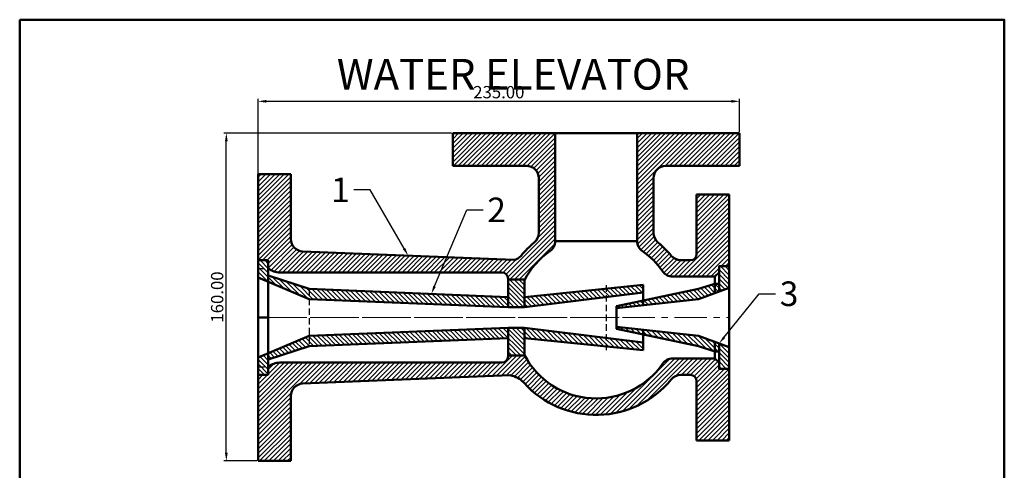
# Model space of a CAD drawing. Units: millimetres. Extents: x 39 to 520, y -165 to 464.
# Tile 4 of 4: x 39 to 520, y 244 to 464. Entities that reach past the tile are written whole.
import ezdxf
from ezdxf import colors
from ezdxf.entities.mleader import LeaderData, LeaderLine
from ezdxf.math import Vec2, Vec3

# ---------------------------------------------------------------- set-up
doc = ezdxf.new("R2010")
doc.units = ezdxf.units.MM
doc.header["$LTSCALE"] = 0.5
doc.linetypes.add('CENTER', pattern=[50.8, 31.75, -6.35, 6.35, -6.35])
doc.linetypes.add('DASHED', pattern=[19.05, 12.7, -6.35])
for name, color, linetype, lineweight in [('M-CNTR', 1, 'CENTER', 18), ('M-DIMS', 2, 'Continuous', 25), ('M-HATC', 8, 'Continuous', 18), ('M-HIDN', 6, 'DASHED', 25), ('M-OUTL', 7, 'Continuous', 50), ('M-TEXT', 3, 'Continuous', 25), ('M-TTLB', 7, 'Continuous', 50)]:
    doc.layers.add(name, color=color, linetype=linetype, lineweight=lineweight)
doc.styles.get("Standard").update_dxf_attribs({"font": 'arial.ttf'})
doc.dimstyles.new('ISO-25', dxfattribs={"dimtxt": 6, "dimasz": 4, "dimexe": 1.25, "dimexo": 0.625, "dimtad": 1, "dimtoh": 1, "dimdec": 1, "dimtxsty": 'Standard', "dimcen": 2.5, "dimadec": 0, "dimazin": 0, "dimtfac": 1, "dimtdec": 1, "dimtofl": 0, "dimtmove": 0, "dimatfit": 3, "dimfxl": 1, "dimarcsym": 0})

# ---------------------------------------------------------------- blocks, each defined once
blk = doc.blocks.new('*D65')
at = {"layer": 'Defpoints', "color": 0, "ltscale": 0.5, "transparency": 16777216}
for p in [(390.62, 424.1), (390.62, 408.6), (155.62, 248.6)]:
    blk.add_point(p, dxfattribs=at)
at = {"layer": 'M-DIMS', "color": 0, "lineweight": -2, "ltscale": 0.5, "transparency": 16777216}
for p, q in [((155.62, 249.23), (155.62, 425.35)), ((159.62, 424.1), (386.62, 424.1)), ((390.62, 409.23), (390.62, 425.35))]:
    blk.add_line(p, q, dxfattribs=at)
at = {"layer": 'M-DIMS', "color": 0, "ltscale": 0.5, "transparency": 16777216}
for points in [[(159.62, 424.77), (159.62, 423.44), (155.62, 424.1)], [(386.62, 424.77), (386.62, 423.44), (390.62, 424.1)]]:
    blk.add_solid(points, dxfattribs=at)
at = {"layer": 'M-DIMS', "color": 0, "ltscale": 0.5, "transparency": 16777216, "insert": (273.12, 427.79), "char_height": 6, "attachment_point": 5}
blk.add_mtext('235.00', dxfattribs=at)
blk = doc.blocks.new('*D66')
at = {"layer": 'Defpoints', "color": 0, "ltscale": 0.5, "transparency": 16777216}
for p in [(140.12, 408.6), (250.62, 408.6), (155.62, 248.6)]:
    blk.add_point(p, dxfattribs=at)
at = {"layer": 'M-DIMS', "color": 0, "lineweight": -2, "ltscale": 0.5, "transparency": 16777216}
for p, q in [((249.99, 408.6), (138.87, 408.6)), ((140.12, 252.6), (140.12, 404.6)), ((154.99, 248.6), (138.87, 248.6))]:
    blk.add_line(p, q, dxfattribs=at)
at = {"layer": 'M-DIMS', "color": 0, "ltscale": 0.5, "transparency": 16777216}
for points in [[(139.45, 404.6), (140.79, 404.6), (140.12, 408.6)], [(139.45, 252.6), (140.79, 252.6), (140.12, 248.6)]]:
    blk.add_solid(points, dxfattribs=at)
at = {"layer": 'M-DIMS', "color": 0, "ltscale": 0.5, "transparency": 16777216, "insert": (136.43, 328.6), "char_height": 6, "attachment_point": 5, "rotation": 90}
blk.add_mtext('160.00', dxfattribs=at)

msp = doc.modelspace()

# ---------------------------------------------------------------- hatches: boundary and pattern name
at = {"layer": 'M-HATC', "ltscale": 0.5}
h = msp.add_hatch(dxfattribs=at)
h.set_pattern_fill('ANSI31', color=256, scale=0.5)
h.set_pattern_definition([(45, (679.1988, 50.7649), (-1.122532, 1.122532), [])])
h.paths.add_polyline_path([(298.0475, 351.0177, 0.24539268), (300.6189, 355.9416), (300.6189, 408.6019), (250.6189, 408.6019), (250.6189, 392.6019), (286.6189, 392.6019, -0.41421356), (292.6189, 386.6019), (292.6189, 359.9087, -0.22417658), (290.432, 355.2762, 0.04839978), (283.9447, 348.7888, -0.17668241), (280.4018, 346.7017), (177.3764, 350.869, -0.40242153), (171.6189, 356.8641), (171.6189, 388.6019), (155.6189, 388.6019), (155.6189, 346.6019), (160.6189, 346.6019), (160.6189, 342.6019, 0.17132661), (166.3069, 340.6019), (274.6189, 340.6019, -0.41421356), (277.6189, 337.6019), (277.6189, 337.1019), (285.7191, 337.1019, -0.11934263)])
h.paths.add_polyline_path([(285.7191, 300.1019), (277.6189, 300.1019), (277.6189, 299.6019, -0.41421356), (274.6189, 296.6019), (166.2844, 296.6019, 0.17068716), (160.6189, 294.6019), (160.6189, 291.1019), (160.6189, 290.6019), (155.6189, 290.6019), (155.6189, 248.6019), (171.6189, 248.6019), (171.6189, 280.3397, -0.40242153), (177.3764, 286.3348), (278.5991, 290.4293, -0.16745848), (285.4544, 286.6692, 0.4573052), (357.2932, 288.415, -0.22417658), (361.9257, 290.6019), (366.6189, 290.6019, -0.41421356), (369.6189, 287.6019), (369.6189, 258.6019), (385.6189, 258.6019), (385.6189, 293.6019), (380.6189, 293.6019), (380.6189, 296.6019), (378.6189, 298.6019), (357.9586, 298.6019, 0.24539268), (353.0347, 296.0305, -0.56130329)])
h.paths.add_polyline_path([(385.6189, 378.6019), (369.6189, 378.6019), (369.6189, 349.6019, -0.41421356), (366.6189, 346.6019), (361.9257, 346.6019, -0.22417658), (357.2932, 348.7888, 0.04839978), (350.8059, 355.2762, -0.22417658), (348.6189, 359.9087), (348.6189, 386.6019, -0.41421356), (354.6189, 392.6019), (390.6189, 392.6019), (390.6189, 408.6019), (340.6189, 408.6019), (340.6189, 355.9416, 0.24539268), (343.1904, 351.0177, -0.08880867), (353.0347, 341.1734, 0.24539268), (357.9586, 338.6019), (378.6189, 338.6019), (380.6189, 340.6019), (380.6189, 343.6019), (385.6189, 343.6019)])
h = msp.add_hatch(dxfattribs=at)
h.set_pattern_fill('ANSI31', color=256, scale=0.5, angle=90)
h.set_pattern_definition([(135, (679.1988, 50.7649), (-1.122532, -1.122532), [])])
h.paths.add_polyline_path([(277.6189, 308.6019), (277.6189, 313.6019), (180.6189, 309.6019), (180.6189, 304.6019)])
h.paths.add_polyline_path([(180.6189, 309.6019), (160.6189, 301.2019), (160.6189, 298.1019), (180.6189, 304.6019)])
h.paths.add_polyline_path([(160.6189, 298.1019), (160.6189, 301.2019), (155.6189, 299.1019), (155.6189, 294.6019), (160.6189, 294.6019)])
h.paths.add_polyline_path([(160.6189, 294.6019), (155.6189, 294.6019), (155.6189, 291.1019), (155.6189, 290.6019), (160.6189, 290.6019)])
h.paths.add_polyline_path([(160.6189, 342.6019), (155.6189, 342.6019), (155.6189, 338.1019), (160.6189, 336.0019)])
h.paths.add_polyline_path([(160.6189, 346.1019), (160.6189, 346.6019), (155.6189, 346.6019), (155.6189, 342.6019), (160.6189, 342.6019)])
h.paths.add_polyline_path([(160.6189, 339.1019), (160.6189, 336.0019), (180.6189, 327.6019), (180.6189, 332.6019)])
h.paths.add_polyline_path([(180.6189, 332.6019), (180.6189, 327.6019), (277.6189, 323.6019), (277.6189, 328.6019)])
h.paths.add_polyline_path([(325.6189, 328.6019), (325.6189, 332.7399), (285.6189, 328.6019), (285.6189, 323.6019)])
h.paths.add_polyline_path([(285.6189, 337.1019), (277.6189, 337.1019), (277.6189, 328.6019), (277.6189, 323.6019), (285.6189, 323.6019), (285.6189, 328.6019)])
h.paths.add_polyline_path([(285.6189, 308.6019), (285.6189, 313.6019), (277.6189, 313.6019), (277.6189, 300.1019), (285.6189, 300.1019)])
h.paths.add_polyline_path([(285.6189, 313.6019), (285.6189, 308.6019), (325.6189, 304.464), (325.6189, 308.6019)])
h.paths.add_polyline_path([(343.6189, 330.8519), (343.6189, 334.6019), (325.6189, 332.7399), (325.6189, 328.6019)])
h.paths.add_polyline_path([(325.6189, 308.6019), (325.6189, 304.464), (343.6189, 302.6019), (343.6189, 306.3519)])
h = msp.add_hatch(dxfattribs=at)
h.set_pattern_fill('ANSI31', color=256, scale=0.5, angle=90)
h.set_pattern_definition([(135, (1020.8346, 209.1737), (-1.122532, -1.122532), [])])
h.paths.add_polyline_path([(370.6189, 327.6019), (385.6189, 333.1019), (385.6189, 343.6019), (380.6189, 343.6019), (380.6189, 335.1019), (378.6189, 335.1019), (370.6189, 332.6019), (330.6189, 324.1019), (330.6189, 323.1019)])
h.paths.add_polyline_path([(378.6189, 302.1019), (380.6189, 302.1019), (380.6189, 293.6019), (385.6189, 293.6019), (385.6189, 304.1019), (370.6189, 309.6019), (330.6189, 314.1019), (330.6189, 313.1019), (370.6189, 304.6019)])

# ---------------------------------------------------------------- linework, layer by layer
at = {"layer": 'M-CNTR'}
msp.add_line((155.6189, 318.6019), (385.6189, 318.6019), dxfattribs=at)
at = {"layer": 'M-CNTR', "ltscale": 0.5}
msp.add_line((155.6189, 318.6019), (343.6189, 318.6019), dxfattribs=at)
at = {"layer": 'M-HIDN', "ltscale": 0.5}
for p, q in [((155.6189, 342.6019), (160.6189, 342.6019)), ((180.6189, 332.6019), (180.6189, 304.6019)), ((325.6189, 302.6019), (325.6189, 334.6019)), ((155.6189, 294.6019), (160.6189, 294.6019))]:
    msp.add_line(p, q, dxfattribs=at)
at = {"layer": 'M-OUTL'}
for p, q in [((320.6189, 408.6019), (250.6189, 408.6019)), ((250.6189, 408.6019), (250.6189, 392.6019)), ((300.6189, 355.9416), (300.6189, 408.6019)), ((390.6189, 408.6019), (320.6189, 408.6019)), ((340.6189, 355.9416), (340.6189, 408.6019)), ((390.6189, 392.6019), (390.6189, 408.6019)), ((250.6189, 392.6019), (286.6189, 392.6019)), ((354.6189, 392.6019), (390.6189, 392.6019)), ((155.6189, 388.6019), (155.6189, 248.6019)), ((171.6189, 388.6019), (155.6189, 388.6019)), ((171.6189, 356.8641), (171.6189, 388.6019)), ((292.6189, 359.9087), (292.6189, 386.6019)), ((348.6189, 359.9087), (348.6189, 386.6019)), ((385.6189, 378.6019), (369.6189, 378.6019)), ((369.6189, 378.6019), (369.6189, 349.6019)), ((385.6189, 318.6019), (385.6189, 378.6019)), ((155.6189, 346.6019), (160.6189, 346.6019)), ((160.6189, 346.6019), (160.6189, 342.6019)), ((361.9257, 346.6019), (366.6189, 346.6019)), ((380.6189, 343.6019), (385.6189, 343.6019)), ((380.6189, 331.2686), (380.6189, 343.6019)), ((166.2844, 340.6019), (274.6189, 340.6019)), ((277.6189, 337.6019), (277.6189, 323.6019)), ((285.6189, 337.1019), (277.6189, 337.1019)), ((285.6189, 323.6019), (285.6189, 337.1019)), ((285.6189, 323.6019), (285.6189, 337.1019)), ((357.9586, 338.6019), (378.6189, 338.6019)), ((378.6189, 338.6019), (380.6189, 340.6019)), ((378.6189, 338.6019), (378.6189, 330.5353)), ((385.6189, 258.6019), (385.6189, 318.6019)), ((277.6189, 313.6019), (277.6189, 299.6019)), ((285.6189, 300.1019), (285.6189, 313.6019)), ((378.6189, 306.6686), (378.6189, 298.6019)), ((380.6189, 296.6019), (380.6189, 305.9353)), ((277.6189, 300.1019), (285.7191, 300.1019)), ((357.9586, 298.6019), (378.6189, 298.6019)), ((378.6189, 298.6019), (380.6189, 296.6019)), ((166.2844, 296.6019), (274.6189, 296.6019)), ((380.6189, 296.6019), (380.6189, 293.6019)), ((380.6189, 293.6019), (385.6189, 293.6019)), ((160.6189, 290.6019), (155.6189, 290.6019)), ((361.9257, 290.6019), (366.6189, 290.6019)), ((369.6189, 287.6019), (369.6189, 258.6019)), ((171.6189, 248.6019), (171.6189, 280.3397)), ((369.6189, 258.6019), (385.6189, 258.6019)), ((155.6189, 248.6019), (171.6189, 248.6019))]:
    msp.add_line(p, q, dxfattribs=at)
at = {"layer": 'M-OUTL', "ltscale": 0.5}
for p, q in [((300.6189, 355.9416), (340.6189, 355.9416)), ((177.3764, 350.869), (280.4018, 346.7017)), ((155.6189, 346.1019), (155.6189, 291.1019)), ((160.6189, 339.1019), (160.6189, 346.1019)), ((155.6189, 318.6019), (155.6189, 342.6019)), ((160.6189, 290.6019), (160.6189, 342.6019)), ((180.6189, 327.6019), (155.6189, 338.1019)), ((160.6189, 339.1019), (180.6189, 332.6019)), ((285.6189, 337.1019), (277.6189, 337.1019)), ((285.6189, 337.1019), (277.6189, 337.1019)), ((277.6189, 337.1019), (277.6189, 328.6019)), ((285.6189, 328.6019), (285.6189, 337.1019)), ((180.6189, 332.6019), (277.6189, 328.6019)), ((285.6189, 328.6019), (343.6189, 334.6019)), ((343.6189, 324.5644), (343.6189, 334.6019)), ((180.6189, 327.6019), (277.6189, 323.6019)), ((285.6189, 323.6019), (343.6189, 330.8519)), ((277.6189, 323.6019), (285.6189, 323.6019)), ((155.6189, 318.6019), (160.6189, 318.6019)), ((180.6189, 309.6019), (277.6189, 313.6019)), ((277.6189, 313.6019), (285.6189, 313.6019)), ((285.6189, 313.6019), (343.6189, 306.3519)), ((343.6189, 302.6019), (343.6189, 312.6394)), ((180.6189, 309.6019), (155.6189, 299.1019)), ((180.6189, 304.6019), (277.6189, 308.6019)), ((277.6189, 308.6019), (277.6189, 300.1019)), ((285.6189, 300.1019), (285.6189, 308.6019)), ((343.6189, 302.6019), (285.6189, 308.6019)), ((160.6189, 298.1019), (180.6189, 304.6019)), ((160.6189, 291.1019), (160.6189, 298.1019)), ((285.6189, 300.1019), (277.6189, 300.1019)), ((177.3764, 286.3348), (278.5991, 290.4293))]:
    msp.add_line(p, q, dxfattribs=at)
msp.add_lwpolyline([(370.6189, 332.6019), (330.6189, 324.1019), (330.6189, 313.1019), (370.6189, 304.6019), (378.6189, 302.1019), (380.6189, 302.1019), (380.6189, 293.6019), (385.6189, 293.6019), (385.6189, 343.6019), (380.6189, 343.6019), (380.6189, 335.1019), (378.6189, 335.1019)], close=True, dxfattribs=at)
for points in [[(385.6189, 333.1019), (370.6189, 327.6019), (330.6189, 323.1019)], [(330.6189, 314.1019), (370.6189, 309.6019), (385.6189, 304.1019)]]:
    msp.add_lwpolyline(points, dxfattribs=at)
at = {"layer": 'M-OUTL'}
for centre, radius, start, end in [((286.6189, 386.6019), 6, 0, 90), ((354.6189, 386.6019), 6, 90, 180), ((286.6189, 359.9087), 6, 309.458119, 0), ((294.6189, 355.9416), 6, 304.849905, 0), ((346.6189, 355.9416), 6, 180, 235.150095), ((354.6189, 359.9087), 6, 180, 230.541881), ((320.6189, 318.6019), 47.5, 129.458119, 140.541881), ((320.6189, 318.6019), 39.5, 124.849905, 152.38422), ((320.6189, 318.6019), 39.5, 34.849905, 55.150095), ((320.6189, 318.6019), 47.5, 39.458119, 50.541881), ((279.3122, 352.6019), 6, 280.462884, 320.541881), ((361.9257, 352.6019), 6, 219.458119, 270), ((366.6189, 349.6019), 3, 270, 0), ((274.6189, 337.6019), 3, 0, 90), ((357.9586, 344.6019), 6, 214.849905, 270), ((274.6189, 299.6019), 3, 270, 0), ((320.6189, 318.6019), 39.5, 207.61578, 325.150095), ((357.9586, 292.6019), 6, 90, 145.150095), ((276.5707, 278.6019), 12, 42.242423, 80.268255), ((320.6189, 318.6019), 47.5, 222.242423, 320.541881), ((361.9257, 284.6019), 6, 90, 140.541881), ((366.6189, 287.6019), 3, 0, 90), ((177.6189, 280.3397), 6, 92.316337, 180)]:
    msp.add_arc(centre, radius, start, end, dxfattribs=at)
at = {"layer": 'M-OUTL', "ltscale": 0.5}
for centre, radius, start, end in [((177.6189, 356.8641), 6, 180, 267.683663), ((166.2957, 349.6582), 9.0563, 231.183581, 270.071194), ((166.2957, 287.5456), 9.0563, 89.928806, 128.816419)]:
    msp.add_arc(centre, radius, start, end, dxfattribs=at)
at = {"layer": 'M-TTLB', "ltscale": 0.5}
msp.add_lwpolyline([(39.27, 463.9335), (519.8288, 463.9335), (519.8288, -165.0878), (39.27, -165.0878)], close=True, dxfattribs=at)

# ---------------------------------------------------------------- texts
at = {"layer": 'M-TEXT', "ltscale": 0.5, "insert": (194.0484, 444.8141), "char_height": 15, "attachment_point": 1}
msp.add_mtext_dynamic_manual_height_columns('WATER ELEVATOR', width=230.78972, gutter_width=12.5, heights=[0], dxfattribs=at)

# ---------------------------------------------------------------- dimensions: what is measured, and where the dimension line sits
at = {"layer": 'M-DIMS', "ltscale": 0.5}
dim = msp.add_linear_dim(base=(390.6189, 424.1019), p1=(155.6189, 248.6019), p2=(390.6189, 408.6019), dimstyle='ISO-25', override={"dimdec": 2, "dimlfac": 1, "dimrnd": 0, "dimzin": 0, "dimdsep": 46, "dimlunit": 2}, dxfattribs=at)
dim.commit()
dim.dimension.update_dxf_attribs({"geometry": '*D65', "text_midpoint": (273.1189, 427.7924)})
dim = msp.add_linear_dim(base=(140.1189, 408.6019), p1=(155.6189, 248.6019), p2=(250.6189, 408.6019), angle=90, dimstyle='ISO-25', override={"dimdec": 2, "dimlfac": 1, "dimrnd": 0, "dimzin": 0, "dimdsep": 46, "dimlunit": 2}, dxfattribs=at)
dim.commit()
dim.dimension.update_dxf_attribs({"geometry": '*D66', "text_midpoint": (136.4305, 328.6019)})

# ---------------------------------------------------------------- leaders
at = {"layer": 'M-TEXT', "ltscale": 0.5}
ml = msp.add_multileader_mtext('Standard', dxfattribs=at)
ml.set_content('1', color=256)
ml.set_leader_properties()
ml.build(insert=Vec2(0, 0))
ctx = ml.context
ctx.base_point, ctx.char_height, ctx.plane_origin = Vec3(193.9252, 380.9041), 12, Vec3(228.8891, 348.7854)
ctx.text_align_type = 2
notes = []
notes.append((ctx, [(0, (1, 1, 0), (210.3454, 380.9041), (-1, 0), 8, [(0, [(228.8891, 348.7854)], 0, [])])]))
ctx.mtext.insert, ctx.mtext.alignment, ctx.mtext.flow_direction = Vec3(200.3454, 386.9041), 3, 5
ml = msp.add_multileader_mtext('Standard', dxfattribs=at)
ml.set_content('2', color=256)
ml.set_leader_properties()
ml.build(insert=Vec2(0, 0))
ctx = ml.context
ctx.base_point, ctx.char_height, ctx.plane_origin = Vec3(265.5047, 371.1397), 12, Vec3(240.1906, 330.1454)
notes.append((ctx, [(0, (1, 1, 0), (257.5047, 371.1397), (1, 0), 8, [(0, [(240.1906, 330.1454)], 0, [])])]))
ctx.mtext.insert, ctx.mtext.flow_direction = Vec3(267.5047, 377.1397), 5
ml = msp.add_multileader_mtext('Standard', dxfattribs=at)
ml.set_content('3', color=256)
ml.set_leader_properties()
ml.build(insert=Vec2(0, 0))
ctx = ml.context
ctx.base_point, ctx.char_height, ctx.plane_origin = Vec3(408.232, 330.1072), 12, Vec3(380.6189, 305.9353)
notes.append((ctx, [(0, (1, 1, 0), (400.232, 330.1072), (1, 0), 8, [(0, [(380.6189, 305.9353)], 0, [])])]))
ctx.mtext.insert, ctx.mtext.flow_direction = Vec3(410.232, 336.2136), 5
for ctx, leaders in notes:
    for number, flags, end, landing, length, lines in leaders:
        leader = LeaderData()
        leader.index, (leader.has_last_leader_line, leader.has_dogleg_vector, leader.attachment_direction) = number, flags
        leader.last_leader_point, leader.dogleg_vector, leader.dogleg_length = Vec3(end), Vec3(landing), length
        for number, points, colour, breaks in lines:
            line = LeaderLine()
            line.index, line.vertices, line.color, line.breaks = number, Vec3.list(points), colors.encode_raw_color(colour), breaks
            leader.lines.append(line)
        ctx.leaders.append(leader)

doc.saveas('drawing.dxf')
